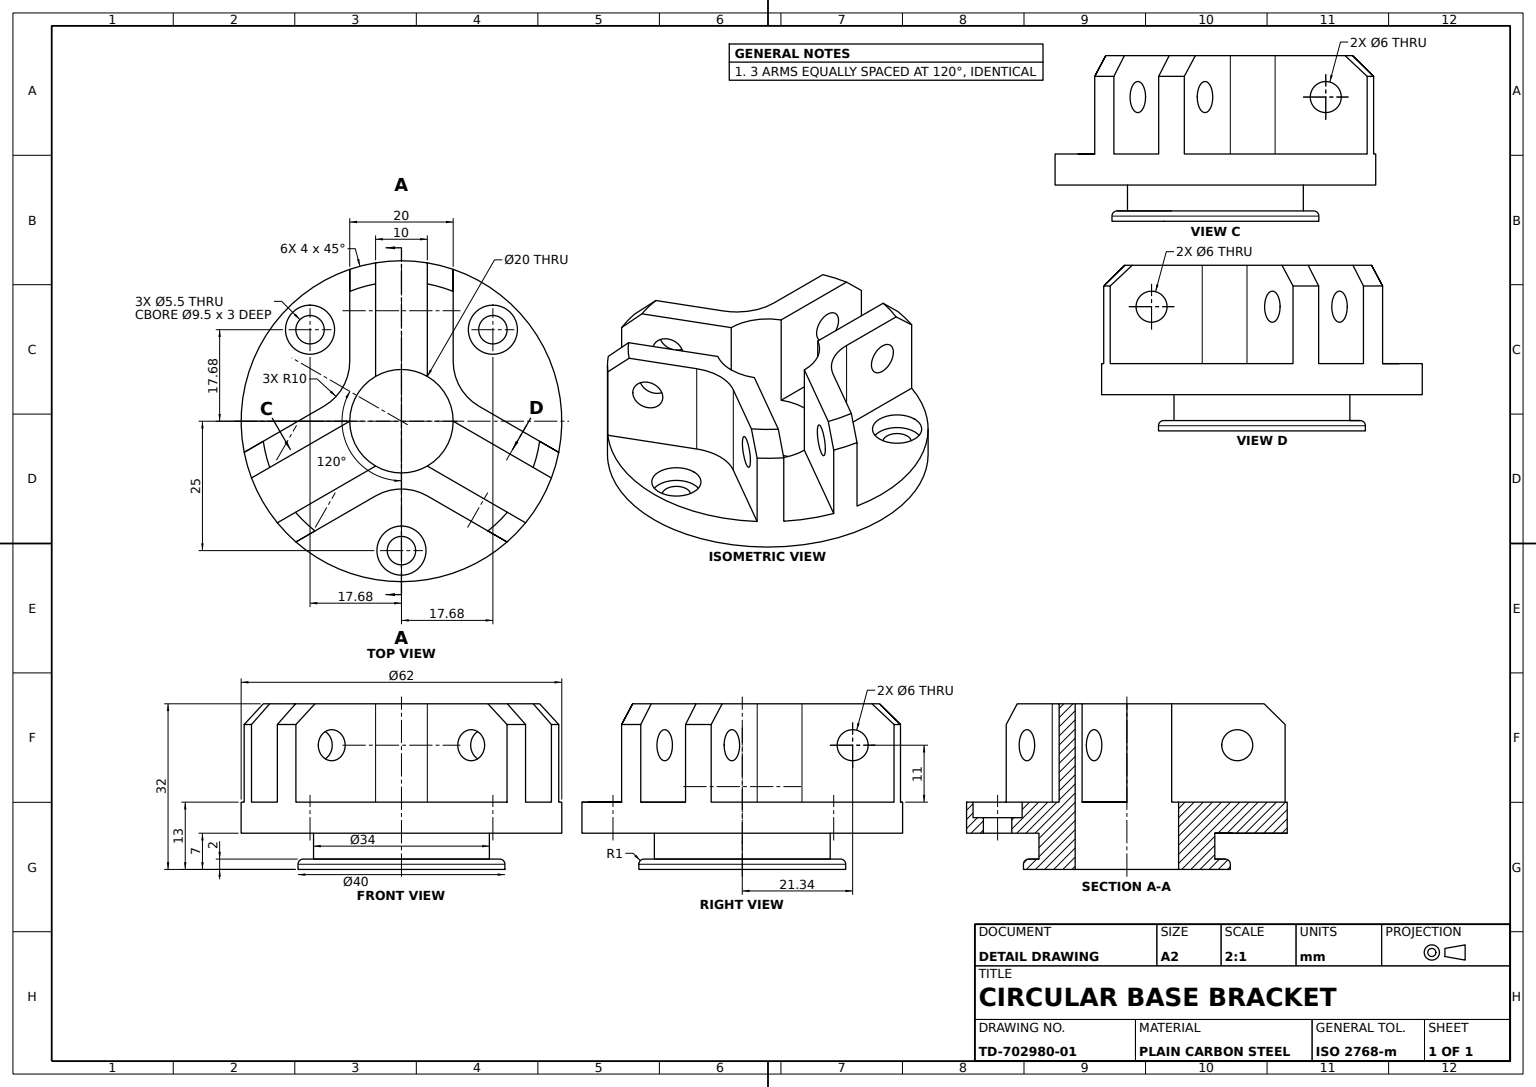
SolidWorks part; units mm, degrees
material "Plain Carbon Steel"
ref_plane "Front Plane" through (0, 0, 0) normal (0, 0, 1) x (1, 0, 0)
ref_plane "Top Plane" through (0, 0, 0) normal (0, 1, 0) x (1, 0, 0)
ref_plane "Right Plane" through (0, 0, 0) normal (1, 0, 0) x (0, 0, -1)
sketch "Base Hub Profile" plane through (0, 0, 0) normal (0, 0, 1) x (1, 0, 0)
  line L0 (0, 0) -> (-20, 0)
  line L1 (-20, 0) -> (-20, 1)
  line L2 (-19, 2) -> (-17, 2)
  line L3 (-17, 2) -> (-17, 7)
  line L4 (-17, 7) -> (-31, 7)
  line L5 (-31, 7) -> (-31, 13)
  line L6 (-31, 13) -> (0, 13)
  line L7 (0, 0) -> (0, 26.52) construction
  line L8 (0, 0) -> (0, 13)
  arc A0 (-19, 2) -> (-20, 1) centre (-19, 1) ccw
  point P12 (-20, 2)
  dimension "D6" = 1
  dimension "D1" = 20
  dimension "D2" = 17
  dimension "D3" = 31
  dimension "D4" = 2
  dimension "D5" = 5
  dimension "D7" = 13
revolve "Base Hub" add sketch "Base Hub Profile" angle 360 about L7
sketch "Arms Profile" plane through (0, 13, 0) normal (0, 1, 0) x (1, 0, 0)
  line L0 (0, 31) -> (0, -5.7735) construction
  line L1 (-31, 0) -> (31, 0) construction
  line L2 (-5, 30.5941) -> (-5, 2.8868)
  line L4 (-10, 29.3428) -> (-10, 5.7735)
  line L5 (5, 30.5941) -> (5, 2.8868)
  line L7 (10, 5.7735) -> (10, 29.3428)
  line L8 (28.9953, -10.9669) -> (5, 2.8868)
  line L10 (30.4116, -6.0111) -> (10, 5.7735)
  line L11 (23.9953, -19.6272) -> (0, -5.7735)
  line L13 (0, -11.547) -> (20.4116, -23.3317)
  line L14 (-23.9953, -19.6272) -> (0, -5.7735)
  line L16 (-20.4116, -23.3317) -> (0, -11.547)
  line L17 (-28.9953, -10.9669) -> (-5, 2.8868)
  line L19 (-10, 5.7735) -> (-30.4116, -6.0111)
  line L24 (0, -10) -> (0, -31) construction
  circle A1 centre (0, 0) radius 31 construction
  arc A3 (10, 29.3428) -> (5, 30.5941) centre (0, 0) ccw
  arc A4 (-5, 30.5941) -> (-10, 29.3428) centre (0, 0) ccw
  arc A5 (20.4116, -23.3317) -> (23.9953, -19.6272) centre (0, 0) ccw
  arc A6 (28.9953, -10.9669) -> (30.4116, -6.0111) centre (0, 0) ccw
  arc A7 (-30.4116, -6.0111) -> (-28.9953, -10.9669) centre (0, 0) ccw
  arc A8 (-23.9953, -19.6272) -> (-20.4116, -23.3317) centre (0, 0) ccw
  point P28 (0, 0)
  point P37 (0, 0)
  point P38 (0, 0)
  dimension "D1" = 10
  dimension "D2" = 5
  dimension "D3" = 10
  dimension "D4" = 5
  dimension "D5" = 10
  dimension "D8" = 120
  dimension "D6" = 2
  dimension "D7" = 2
extrude "Three Arms" add sketch "Arms Profile" along normal blind 19
sketch "Centre Bore Sketch" plane through (0, 0, 0) normal (0, -1, 0) x (1, 0, 0)
  circle A0 centre (0, 0) radius 10
  dimension "D1" = 20
extrude "Centre Bore" cut sketch "Centre Bore Sketch" against normal blind 79
fillet "Arm Fillets R10 A" radius 10 1 edges at (-10, 22.5, -5.7735)
fillet "Arm Fillets R10 B" radius 10 2 edges at (10, 22.5, -5.7735) (0, 22.5, 11.547)
sketch "Arm Hole 1 Sketch" plane through (5, 0, 8.6603) normal (0.5, 0, 0.866) x (0.866, 0, -0.5)
  line L0 (6.0111, 13) -> (-29.3428, 13) construction
  line L1 (-29.3428, 32) -> (-29.3428, 13) construction
  circle A0 centre (-21.3428, 24) radius 3
  dimension "D1" = 6
  dimension "D2" = 11
  dimension "D3" = 8
extrude "Arm Hole 1" cut sketch "Arm Hole 1 Sketch" against normal blind 79
sketch "Arm Hole 2 Sketch" plane through (-10, 0, 0) normal (-1, 0, 0) x (0, 0, 1)
  line L0 (-29.3428, 13) -> (-11.547, 13) construction
  line L1 (-29.3428, 32) -> (-29.3428, 13) construction
  circle A0 centre (-21.3428, 24) radius 3
  dimension "D3" = 6
  dimension "D1" = 11
  dimension "D2" = 8
extrude "Arm Hole 2" cut sketch "Arm Hole 2 Sketch" against normal blind 79
sketch "Arm Hole 3 Sketch" plane through (5, 0, -8.6603) normal (0.5, 0, -0.866) x (-0.866, 0, -0.5)
  line L0 (-29.3428, 13) -> (-11.547, 13) construction
  line L1 (-29.3428, 32) -> (-29.3428, 13) construction
  circle A0 centre (-21.3428, 24) radius 3
  dimension "D3" = 6
  dimension "D1" = 11
  dimension "D2" = 8
extrude "Arm Hole 3" cut sketch "Arm Hole 3 Sketch" against normal blind 79
chamfer "Arm Chamfer 4mm" distance 4 angle 45 6 edges at (29.8066, 32, 8.5185) (22.2806, 32, 21.554) (-22.2806, 32, 21.554) (-29.8066, 32, 8.5185) (-7.5261, 32, -30.0726) (7.5261, 32, -30.0726)
sketch "Base Hole Positions" plane through (0, 13, 0) normal (0, 1, 0) x (1, 0, 0)
  line L0 (-31, 0) -> (31, 0) construction
  line L2 (0, -25) -> (0, 31) construction
  line L3 (0, 31) -> (0, 0) construction
  line L4 (0, 0) -> (-17.6777, 17.6777) construction
  line L5 (-17.6777, 17.6777) -> (17.6777, -17.6777) construction
  line L6 (17.6777, -17.6777) -> (0, 0) construction
  line L7 (0, 0) -> (-17.6777, -17.6777) construction
  line L8 (-17.6777, -17.6777) -> (17.6777, 17.6777) construction
  circle A0 centre (0, 0) radius 25 construction
  arc A1 (-10, 29.3428) -> (-30.4116, -6.0111) centre (0, 0) ccw construction
  arc A2 (30.4116, -6.0111) -> (10, 29.3428) centre (0, 0) ccw construction
  arc A4 (5, 30.5941) -> (-5, 30.5941) centre (0, 0) ccw construction
  dimension "D1" = 50
  dimension "D2" = 45
  dimension "D3" = 45
  dimension "D4" = 45
  dimension "D5" = 45
  dimension "D6" = 45
hole_wizard "Base C-Bore Holes Ø5.5" positions "Sketch14" profile "Sketch15" legacy
sketch "Sketch14" plane through (0, 13, 0) normal (0, 1, 0) x (1, 0, 0)
  point P0 (-17.6777, 17.6777)
  point P3 (0, -25)
  point P6 (17.6777, 17.6777)
sketch "Sketch15" plane through (-17.6777, 13, -17.6777) normal (1, 0, 0) x (0, 0, 1)
  line L0 (0, 0) -> (0, 9)
  line L1 (0, 9) -> (2.75, 9)
  line L2 (2.75, 9) -> (2.75, 3)
  line L3 (2.75, 3) -> (4.75, 3)
  line L4 (4.75, 3) -> (4.75, 0)
  line L5 (4.75, 0) -> (0, 0)
  line L6 (0, 110) -> (0, -10) construction
  dimension "Diameter" = 5.5
  dimension "Depth" = 9
  dimension "C-Bore Diameter" = 9.5
  dimension "C-Bore Depth" = 3
